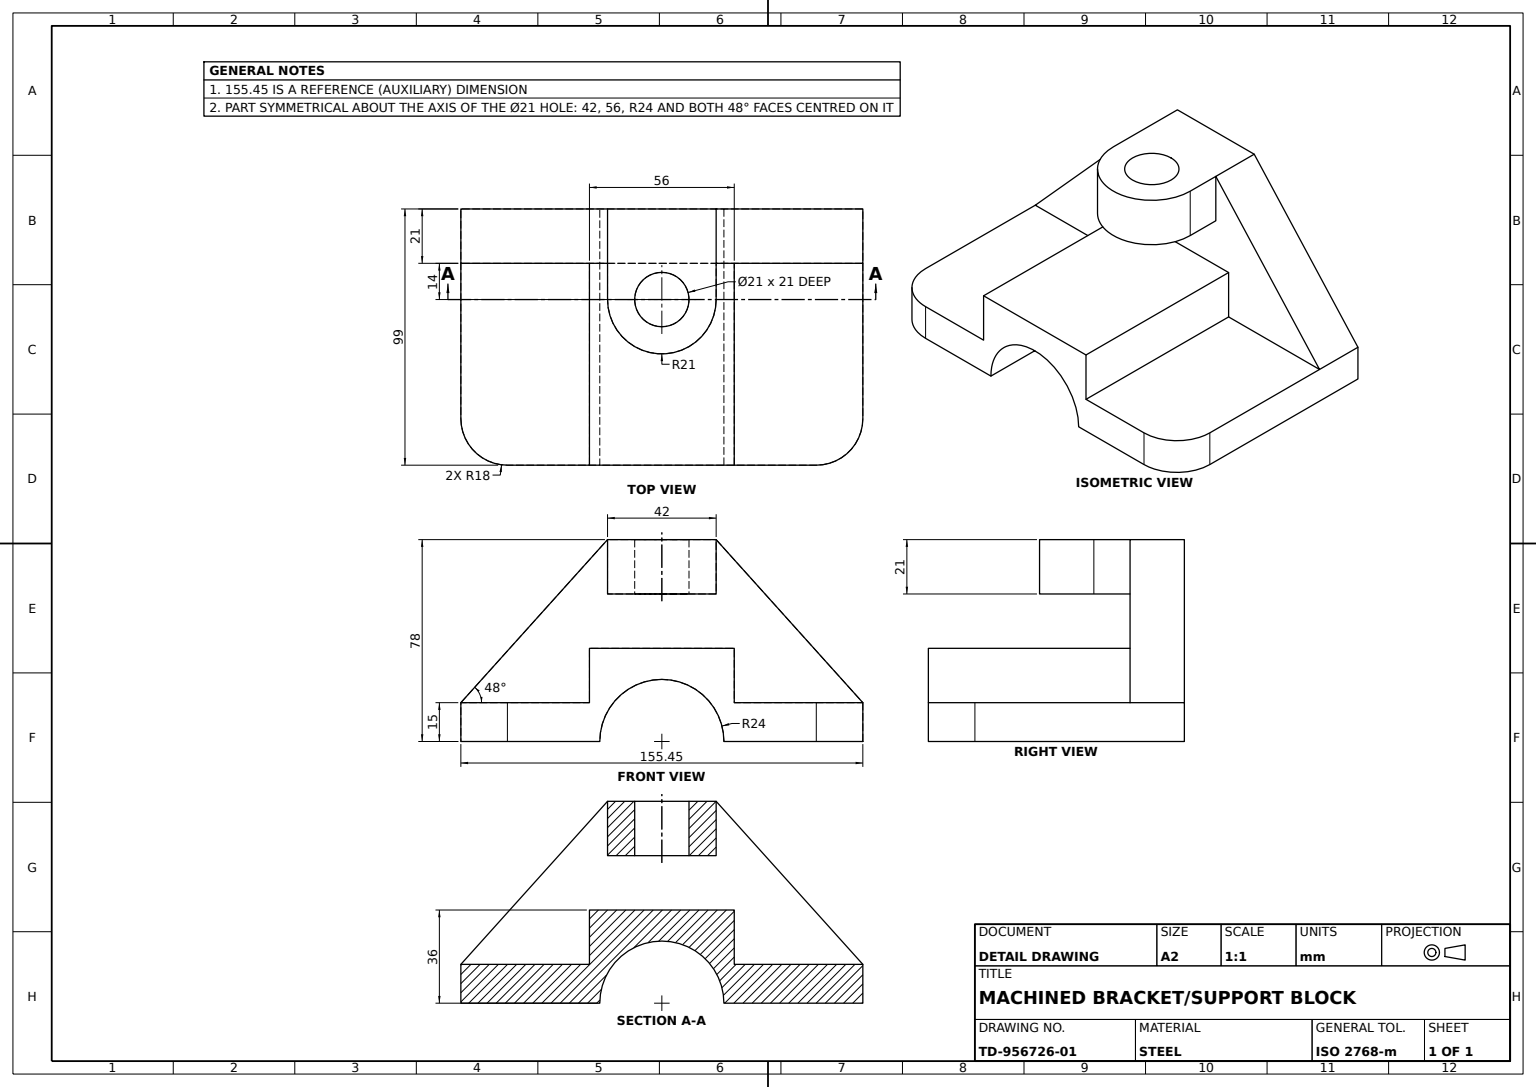
from build123d import *

# Parameters (mm, degrees)
BASE_PLATE_SKETCH_R     = 10.5
BASE_PLATE_DEPTH        = 21
ANGLED_WEB_48DEG_DEPTH  = 21
UPRIGHT_BLOCK_DEPTH     = 78
CORNER_FILLETS_R18_R    = 18
HALF_ROUND_CUT_24_REACH = 140.171


with BuildPart() as part:
    # Base Plate Sketch → Base Plate (new body)
    with BuildSketch(Plane(origin=(0, 0, 0), x_dir=(1, 0, 0), z_dir=(0, 1, 0))):
        with BuildLine():
            Line((-21, 0), (-21, 35))
            Line((-21, 35), (21, 35))
            Line((21, 35), (21, 0))
            ThreePointArc((21, 0), (0, -21), (-21, 0))
        make_face()
        with Locations(Location((0, 0, 0), (0, 0, 90))):
            Circle(BASE_PLATE_SKETCH_R, mode=Mode.SUBTRACT)
    extrude(amount=BASE_PLATE_DEPTH)

    # Angled Web Sketch → Angled Web 48deg (add)
    with BuildSketch(Plane(origin=(0, 0, -35), x_dir=(-1, 0, 0), z_dir=(0, 0, -1))):
        Polygon((77.725454791, -42), (77.725454791, -57), (-77.725454791, -57), (-77.725454791, -42), (-21, 21), (21, 21), align=None)
    extrude(amount=-ANGLED_WEB_48DEG_DEPTH)

    # Upright Block Sketch → Upright Block (add)
    with BuildSketch(Plane.XY.offset(-14)):
        Polygon((-77.725454791, -42), (-28, -42), (-28, -21), (28, -21), (28, -42), (77.725454791, -42), (77.725454791, -57), (-77.725454791, -57), align=None)
    extrude(amount=UPRIGHT_BLOCK_DEPTH)

    # Corner Fillets R18
    corner_fillets_r18_edges = [part.edges().sort_by_distance(p)[0] for p in [
        (-77.725454791, -49.5, 64),
        (77.725454791, -49.5, 64),
    ]]
    fillet(corner_fillets_r18_edges, radius=CORNER_FILLETS_R18_R)

    # Half-Round Cut Sketch → Half-Round Cut Ø24 (cut, up to next)
    with BuildSketch(Plane.XY.offset(64), mode=Mode.PRIVATE) as half_round_cut_24_sk1:
        with BuildLine():
            Line((-24, -57), (24, -57))
            ThreePointArc((24, -57), (0, -33), (-24, -57))
        make_face()
    half_round_cut_24_tool1 = extrude(half_round_cut_24_sk1.sketch, amount=-HALF_ROUND_CUT_24_REACH, mode=Mode.PRIVATE) & part.part
    add(half_round_cut_24_tool1.solids().sort_by_distance((0, -46.814084, 64))[0], mode=Mode.SUBTRACT)


solid = part.part
